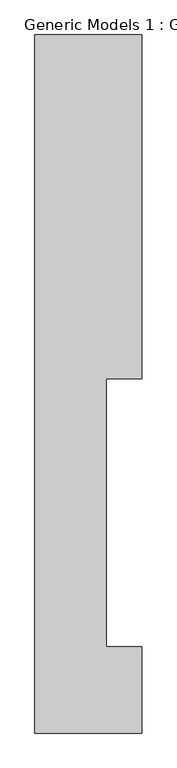
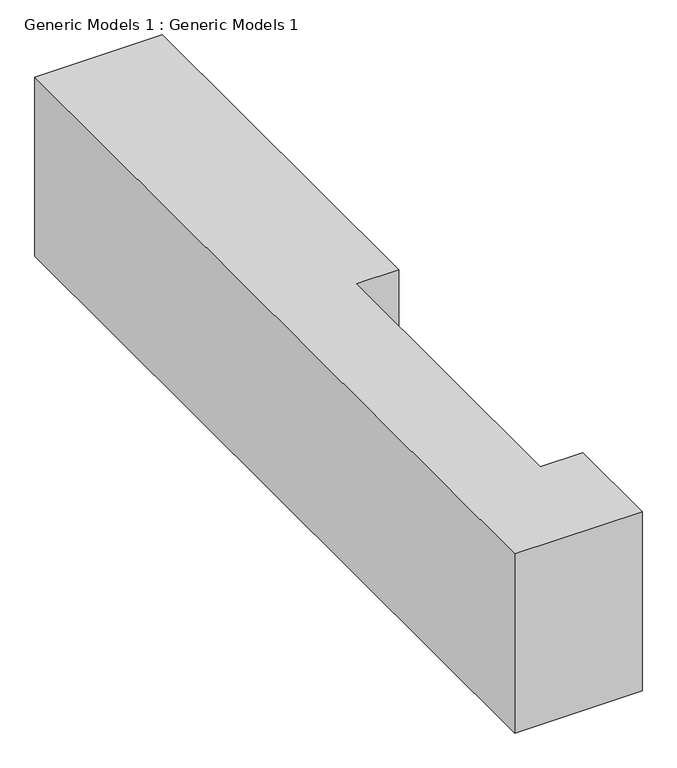
"""IFC4 building model written with IfcOpenShell, lengths in millimetres: proxy geometry, Generic Models 1 : Generic Models 1."""

from ifc_helpers import new_model, si_unit, frame, origin, place, context, project, spatial, polyline, outline, extrude, source, transform, mapped, element, save


def generic_models_1_generic_models_1_9f30b8ca(model_context):
    return source(origin(), model_context, "Body", "SweptSolid", [
        extrude(outline(polyline([(-9259.9126504, 2117.2946558), (-8345.5126504, 2117.2946558), (-8345.5126504, -821.2447089), (-8650.3126504, -821.2447089), (-8650.3126504, -3109.5857243), (-8345.5126504, -3109.5857243), (-8345.5126504, -3847.271143), (-9259.9126504, -3847.271143), (-9259.9126504, 2117.2946558)])), frame((0.0, 0.0, 582.9900954), z_axis=(0.0, 0.0, 1.0), x_axis=(1.0, 0.0, 0.0)), (0.0, 0.0, 1.0), 1361.0905882),
    ])


if __name__ == "__main__":
    model = new_model("IFC4")
    model_context = context("Model", 3, world=origin())
    ifc_project = project(units=[si_unit("LENGTHUNIT", "METRE", prefix="MILLI")], contexts=[model_context])
    site = spatial("IfcSite", under=ifc_project)
    building = spatial("IfcBuilding", under=site)
    placement = place(None, origin())
    generic_models_1_generic_models_1_shape = generic_models_1_generic_models_1_9f30b8ca(model_context)
    element("IfcBuildingElementProxy", 1, Name="Generic Models 1 : Generic Models 1", ObjectType="Generic Models 1 : Generic Models 1", at=placement, inside=building, context=model_context, shape_type="MappedRepresentation", body=[
        mapped(generic_models_1_generic_models_1_shape, transform((0.0, 0.0, 0.0), x_axis=(1.0, 0.0, 0.0), y_axis=(0.0, 1.0, 0.0), z_axis=(0.0, 0.0, 1.0))),
    ])
    save(model, "model.ifc")
